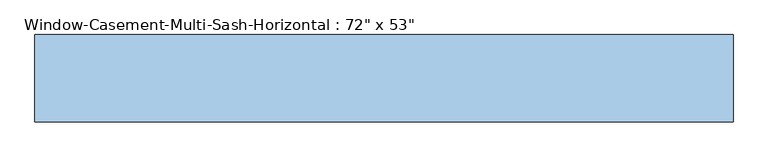
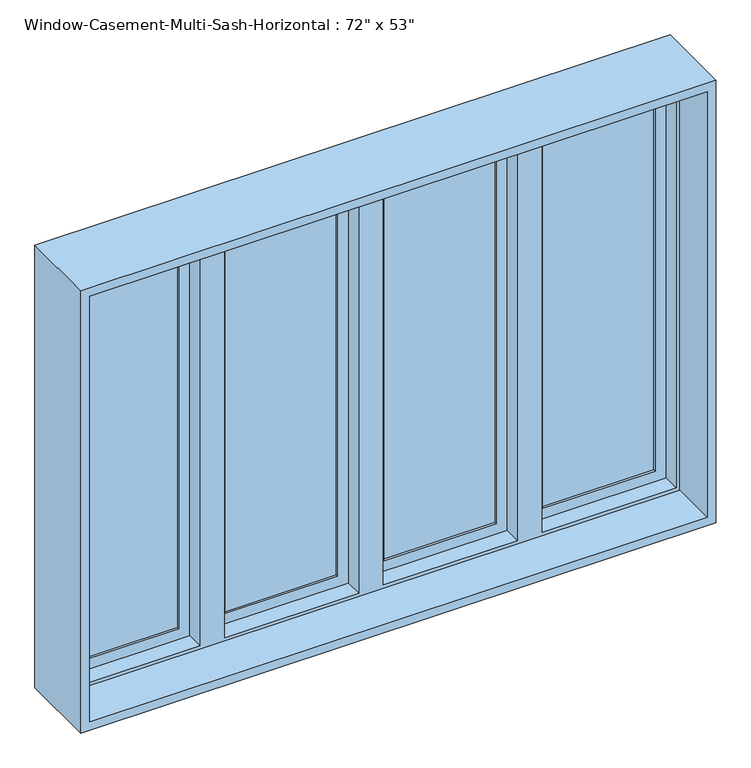
"""IFC4 building model written with IfcOpenShell, lengths in millimetres: window geometry."""

from ifc_helpers import new_model, si_unit, frame, origin, place, context, project, spatial, polyline, outline, extrude, faceted_brep, source, transform, mapped, element, save


def window_5487fb6d(model_context):
    return source(origin(), model_context, "Body", "SolidModel", [
        extrude(outline(polyline([(2235.2, 482.6), (939.8, 482.6), (939.8, 889.0), (2235.2, 889.0), (2235.2, 482.6)]), holes=[polyline([(2193.3296875, 847.1296875), (981.6703125, 847.1296875), (981.6703125, 524.4703125), (2193.3296875, 524.4703125), (2193.3296875, 847.1296875)])]), frame((0.0, 73.025, 0.0), z_axis=(0.0, 1.0, 0.0), x_axis=(0.0, 0.0, 1.0)), (0.0, 0.0, 1.0), 31.75),
        extrude(outline(polyline([(2235.2, -889.0), (939.8, -889.0), (939.8, -482.6), (2235.2, -482.6), (2235.2, -889.0)]), holes=[polyline([(2193.3296875, -524.4703125), (981.6703125, -524.4703125), (981.6703125, -847.1296875), (2193.3296875, -847.1296875), (2193.3296875, -524.4703125)])]), frame((0.0, 73.025, 0.0), z_axis=(0.0, 1.0, 0.0), x_axis=(0.0, 0.0, 1.0)), (0.0, 0.0, 1.0), 31.75),
        extrude(outline(polyline([(-524.4703125, 98.425), (-524.4703125, 92.075), (-847.1296875, 92.075), (-847.1296875, 98.425), (-524.4703125, 98.425)])), frame((0.0, 0.0, 981.6703125), z_axis=(0.0, 0.0, 1.0), x_axis=(1.0, 0.0, 0.0)), (0.0, 0.0, 1.0), 1211.659375),
        extrude(outline(polyline([(-524.4703125, 85.725), (-524.4703125, 79.375), (-847.1296875, 79.375), (-847.1296875, 85.725), (-524.4703125, 85.725)])), frame((0.0, 0.0, 981.6703125), z_axis=(0.0, 0.0, 1.0), x_axis=(1.0, 0.0, 0.0)), (0.0, 0.0, 1.0), 1211.659375),
        extrude(outline(polyline([(847.1296875, 98.425), (847.1296875, 92.075), (524.4703125, 92.075), (524.4703125, 98.425), (847.1296875, 98.425)])), frame((0.0, 0.0, 981.6703125), z_axis=(0.0, 0.0, 1.0), x_axis=(1.0, 0.0, 0.0)), (0.0, 0.0, 1.0), 1211.659375),
        extrude(outline(polyline([(847.1296875, 85.725), (847.1296875, 79.375), (524.4703125, 79.375), (524.4703125, 85.725), (847.1296875, 85.725)])), frame((0.0, 0.0, 981.6703125), z_axis=(0.0, 0.0, 1.0), x_axis=(1.0, 0.0, 0.0)), (0.0, 0.0, 1.0), 1211.659375),
        extrude(outline(polyline([(-67.2703125, 98.425), (-67.2703125, 92.075), (-389.9296875, 92.075), (-389.9296875, 98.425), (-67.2703125, 98.425)])), frame((0.0, 0.0, 981.6703125), z_axis=(0.0, 0.0, 1.0), x_axis=(1.0, 0.0, 0.0)), (0.0, 0.0, 1.0), 1211.659375),
        extrude(outline(polyline([(-67.2703125, 85.725), (-67.2703125, 79.375), (-389.9296875, 79.375), (-389.9296875, 85.725), (-67.2703125, 85.725)])), frame((0.0, 0.0, 981.6703125), z_axis=(0.0, 0.0, 1.0), x_axis=(1.0, 0.0, 0.0)), (0.0, 0.0, 1.0), 1211.659375),
        extrude(outline(polyline([(389.9296875, 98.425), (389.9296875, 92.075), (67.2703125, 92.075), (67.2703125, 98.425), (389.9296875, 98.425)])), frame((0.0, 0.0, 981.6703125), z_axis=(0.0, 0.0, 1.0), x_axis=(1.0, 0.0, 0.0)), (0.0, 0.0, 1.0), 1211.659375),
        extrude(outline(polyline([(389.9296875, 85.725), (389.9296875, 79.375), (67.2703125, 79.375), (67.2703125, 85.725), (389.9296875, 85.725)])), frame((0.0, 0.0, 981.6703125), z_axis=(0.0, 0.0, 1.0), x_axis=(1.0, 0.0, 0.0)), (0.0, 0.0, 1.0), 1211.659375),
        faceted_brep([(-482.6, 73.025, 2235.2), (-889.0, 73.025, 2235.2), (-889.0, 114.3, 2235.2), (889.0, 114.3, 2235.2), (889.0, 73.025, 2235.2), (482.6, 73.025, 2235.2), (482.6, 111.125, 2235.2), (431.8, 111.125, 2235.2), (431.8, 73.025, 2235.2), (25.4, 73.025, 2235.2), (25.4, 111.125, 2235.2), (-25.4, 111.125, 2235.2), (-25.4, 73.025, 2235.2), (-431.8, 73.025, 2235.2), (-431.8, 111.125, 2235.2), (-482.6, 111.125, 2235.2), (-878.8796875, 22.225, 2225.0796875), (-878.8796875, 73.025, 2225.0796875), (-492.7203125, 73.025, 2225.0796875), (-492.7203125, 22.225, 2225.0796875), (878.8796875, 73.025, 2225.0796875), (878.8796875, 22.225, 2225.0796875), (492.7203125, 22.225, 2225.0796875), (492.7203125, 73.025, 2225.0796875), (-421.6796875, 73.025, 2225.0796875), (-35.5203125, 73.025, 2225.0796875), (-35.5203125, 22.225, 2225.0796875), (-421.6796875, 22.225, 2225.0796875), (35.5203125, 73.025, 2225.0796875), (421.6796875, 73.025, 2225.0796875), (421.6796875, 22.225, 2225.0796875), (35.5203125, 22.225, 2225.0796875), (-889.0, -114.3, 2235.2), (-889.0, 22.225, 2235.2), (889.0, 22.225, 2235.2), (889.0, -114.3, 2235.2), (-914.4, 114.3, 2260.6), (-914.4, -114.3, 2260.6), (914.4, -114.3, 2260.6), (914.4, 114.3, 2260.6), (889.0, 114.3, 939.8), (889.0, 73.025, 939.8), (878.8796875, 73.025, 949.9203125), (878.8796875, 22.225, 949.9203125), (889.0, 22.225, 939.8), (889.0, -114.3, 939.8), (914.4, -114.3, 914.4), (914.4, 114.3, 914.4), (482.6, 73.025, 939.8), (-889.0, 114.3, 939.8), (-889.0, 73.025, 939.8), (-482.6, 73.025, 939.8), (-482.6, 111.125, 939.8), (-431.8, 111.125, 939.8), (-431.8, 73.025, 939.8), (-25.4, 73.025, 939.8), (-25.4, 111.125, 939.8), (25.4, 111.125, 939.8), (25.4, 73.025, 939.8), (431.8, 73.025, 939.8), (431.8, 111.125, 939.8), (482.6, 111.125, 939.8), (492.7203125, 73.025, 949.9203125), (492.7203125, 22.225, 949.9203125), (-878.8796875, 73.025, 949.9203125), (-878.8796875, 22.225, 949.9203125), (-492.7203125, 22.225, 949.9203125), (-492.7203125, 73.025, 949.9203125), (-35.5203125, 73.025, 949.9203125), (-421.6796875, 73.025, 949.9203125), (-421.6796875, 22.225, 949.9203125), (-35.5203125, 22.225, 949.9203125), (421.6796875, 73.025, 949.9203125), (35.5203125, 73.025, 949.9203125), (35.5203125, 22.225, 949.9203125), (421.6796875, 22.225, 949.9203125), (-889.0, 22.225, 939.8), (-889.0, -114.3, 939.8), (-914.4, -114.3, 914.4), (-914.4, 114.3, 914.4)], [[[0, 1, 2, 3, 4, 5, 6, 7, 8, 9, 10, 11, 12, 13, 14, 15]], [[16, 17, 18, 19]], [[20, 21, 22, 23]], [[24, 25, 26, 27]], [[28, 29, 30, 31]], [[32, 33, 34, 35]], [[36, 37, 38, 39]], [[4, 3, 40, 41]], [[21, 20, 42, 43]], [[35, 34, 44, 45]], [[39, 38, 46, 47]], [[48, 41, 40, 49, 50, 51, 52, 53, 54, 55, 56, 57, 58, 59, 60, 61]], [[43, 42, 62, 63]], [[64, 65, 66, 67]], [[68, 69, 70, 71]], [[72, 73, 74, 75]], [[45, 44, 76, 77]], [[47, 46, 78, 79]], [[2, 1, 50, 49]], [[4, 41, 48, 5], [20, 23, 62, 42]], [[50, 1, 0, 51], [64, 67, 18, 17]], [[12, 55, 54, 13], [69, 68, 25, 24]], [[8, 59, 58, 9], [73, 72, 29, 28]], [[17, 16, 65, 64]], [[44, 34, 33, 76], [16, 19, 66, 65], [27, 26, 71, 70], [31, 30, 75, 74], [21, 43, 63, 22]], [[33, 32, 77, 76]], [[38, 37, 78, 46], [32, 35, 45, 77]], [[37, 36, 79, 78]], [[36, 39, 47, 79], [3, 2, 49, 40]], [[18, 67, 66, 19]], [[69, 24, 27, 70]], [[53, 14, 13, 54]], [[14, 53, 52, 15]], [[15, 52, 51, 0]], [[25, 68, 71, 26]], [[73, 28, 31, 74]], [[57, 10, 9, 58]], [[10, 57, 56, 11]], [[11, 56, 55, 12]], [[6, 61, 60, 7]], [[7, 60, 59, 8]], [[29, 72, 75, 30]], [[62, 23, 22, 63]], [[61, 6, 5, 48]]]),
        extrude(outline(polyline([(2235.2, 25.4), (939.8, 25.4), (939.8, 431.8), (2235.2, 431.8), (2235.2, 25.4)]), holes=[polyline([(2193.3296875, 389.9296875), (981.6703125, 389.9296875), (981.6703125, 67.2703125), (2193.3296875, 67.2703125), (2193.3296875, 389.9296875)])]), frame((0.0, 73.025, 0.0), z_axis=(0.0, 1.0, 0.0), x_axis=(0.0, 0.0, 1.0)), (0.0, 0.0, 1.0), 31.75),
        extrude(outline(polyline([(2235.2, -431.8), (939.8, -431.8), (939.8, -25.4), (2235.2, -25.4), (2235.2, -431.8)]), holes=[polyline([(2193.3296875, -67.2703125), (981.6703125, -67.2703125), (981.6703125, -389.9296875), (2193.3296875, -389.9296875), (2193.3296875, -67.2703125)])]), frame((0.0, 73.025, 0.0), z_axis=(0.0, 1.0, 0.0), x_axis=(0.0, 0.0, 1.0)), (0.0, 0.0, 1.0), 31.75),
    ])


if __name__ == "__main__":
    model = new_model("IFC4")
    model_context = context("Model", 3, world=origin())
    ifc_project = project(units=[si_unit("LENGTHUNIT", "METRE", prefix="MILLI")], contexts=[model_context])
    site = spatial("IfcSite", under=ifc_project)
    building = spatial("IfcBuilding", under=site)
    placement = place(None, origin())
    window_shape = window_5487fb6d(model_context)
    element("IfcWindow", 1, ObjectType="Window-Casement-Multi-Sash-Horizontal : 72\" x 53\"", at=placement, inside=building, context=model_context, shape_type="MappedRepresentation", body=[
        mapped(window_shape, transform((0.0, 0.0, 0.0), x_axis=(1.0, 0.0, 0.0), y_axis=(0.0, 1.0, 0.0), z_axis=(0.0, 0.0, 1.0))),
    ])
    save(model, "model.ifc")

# Revit data of these elements
# Type "Window-Casement-Multi-Sash-Horizontal : 72\" x 53\""
#   Type Mark = "23"
#   Fire Rating = "0.5h"
#   Assembly Code = "B2020100"
#   Analytic Construction = "Double glazing - domestic"
#   Window Inset [instance default] = 0.052083 ft
#   Wall Thickness [instance default] = 0.5 ft
#   Visual Light Transmittance = 0.81
#   Thermal Resistance (R) = 1.8146 (h·ft²·°F)/BTU
#   Solar Heat Gain Coefficient = 0.76
#   Rough Width = 6.041667 ft
#   Rough Height = 4.458333 ft
#   Open Window Width = 1.5 ft
#   Heat Transfer Coefficient (U) = 0.5511 BTU/(h·ft²·°F)
#   Height = 4.416667 ft
#   Frame Gap 3 [instance default] = 0.13737 ft
#   Frame Gap 2 [instance default] = 0.052083 ft
#   Frame Gap 1 = 0.116536 ft
#   Default Sill Height = 3 ft
#   Width = 6 ft
#   Frame Material = Metal - Aluminum
#   Glass Panel Material = Glass
#   Wall Closure = (empty or 0)
# Element 1 (IfcWindow, "Window-Casement-Multi-Sash-Horizontal : 72\" x 53\"")
#   Wall Thickness = 0.75 ft
#   Materials on its faces: "Metal - Aluminum", "Glass"
# Materials
#   "Metal - Aluminum": class "Metal", colour RGB 247 247 247, transparency 0
#   "Glass": class "Glass", colour RGB 0 128 192, transparency 0.75, Description = "Soda Lime Glass", Cost = 0
